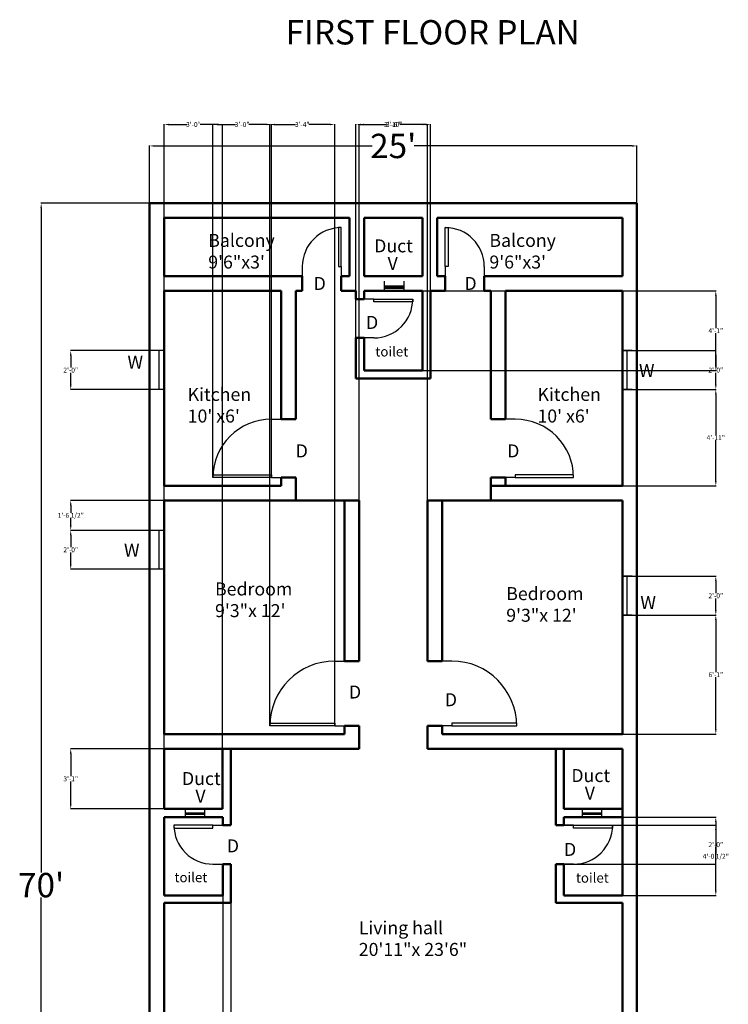
# Model space of a CAD drawing. Units: inches. Extents: x -250 to 2650, y 180 to 1183.
# Tile 4 of 10: x 296 to 732, y 577 to 1183. Entities that reach past the tile are written whole.
import ezdxf

# ---------------------------------------------------------------- set-up
doc = ezdxf.new("R2010")
doc.units = ezdxf.units.IN
doc.header["$MEASUREMENT"] = 0
for name, color, linetype, lineweight in [('A-ANNO-DIMS', 2, 'Continuous', 18), ('A-ANNO-TEXT', 7, 'Continuous', 18), ('A-AREA-IDEN', 3, 'Continuous', 18), ('A-DOOR', 4, 'Continuous', 25), ('A-GLAZ', 3, 'Continuous', 25), ('A-WALL', 7, 'Continuous', 50)]:
    doc.layers.add(name, color=color, linetype=linetype, lineweight=lineweight)
doc.styles.get("Standard").update_dxf_attribs({"font": 'arial.ttf'})
doc.dimstyles.get("Standard").update_dxf_attribs({"dimtxt": 3, "dimasz": 3, "dimexe": 0.18, "dimexo": 0.0625, "dimgap": 0.09, "dimtad": 0, "dimtih": 1, "dimtoh": 1, "dimdec": 0, "dimzin": 0, "dimdsep": 46, "dimlunit": 3, "dimtxsty": 'Standard', "dimcen": 0.09, "dimadec": 0, "dimazin": 0, "dimtfac": 1, "dimtdec": 0, "dimtofl": 0, "dimtmove": 0, "dimatfit": 3, "dimfxl": 1, "dimtolj": 1, "dimtzin": 0, "dimarcsym": 0})

# ---------------------------------------------------------------- blocks, each defined once
blk = doc.blocks.new('*D15')
at = {"layer": 'A-ANNO-DIMS', "color": 0, "lineweight": -2, "transparency": 16777216}
for p, q in [((376.08, 1070.09), (376.08, 1105.5)), ((379.08, 1105.32), (513.14, 1105.32)), ((673.08, 1105.32), (539.03, 1105.32)), ((676.08, 1070.09), (676.08, 1105.5))]:
    blk.add_line(p, q, dxfattribs=at)
at = {"layer": 'A-ANNO-DIMS', "color": 0, "transparency": 16777216}
for points in [[(379.08, 1105.82), (379.08, 1104.82), (376.08, 1105.32)], [(673.08, 1105.82), (673.08, 1104.82), (676.08, 1105.32)]]:
    blk.add_solid(points, dxfattribs=at)
at = {"layer": 'Defpoints', "color": 0, "transparency": 16777216}
for p in [(376.08, 1105.32), (376.08, 1070.02), (676.08, 1070.02)]:
    blk.add_point(p, dxfattribs=at)
at = {"layer": 'A-ANNO-DIMS', "color": 0, "transparency": 16777216, "insert": (526.08, 1105.32), "char_height": 3, "attachment_point": 5}
blk.add_mtext("\\A1;{\\H5x;25'}", dxfattribs=at)
blk = doc.blocks.new('*D16')
at = {"layer": 'A-ANNO-DIMS', "color": 0, "lineweight": -2, "transparency": 16777216}
for p, q in [((376.02, 1070.02), (309.2, 1070.02)), ((309.38, 1067.02), (309.38, 657.77)), ((309.38, 233.02), (309.38, 642.28)), ((376.02, 230.02), (309.2, 230.02))]:
    blk.add_line(p, q, dxfattribs=at)
at = {"layer": 'A-ANNO-DIMS', "color": 0, "transparency": 16777216}
for points in [[(308.88, 1067.02), (309.88, 1067.02), (309.38, 1070.02)], [(308.88, 233.02), (309.88, 233.02), (309.38, 230.02)]]:
    blk.add_solid(points, dxfattribs=at)
at = {"layer": 'Defpoints', "color": 0, "transparency": 16777216}
for p in [(376.08, 1070.02), (309.38, 230.02), (376.08, 230.02)]:
    blk.add_point(p, dxfattribs=at)
at = {"layer": 'A-ANNO-DIMS', "color": 0, "transparency": 16777216, "insert": (309.38, 650.02), "char_height": 3, "attachment_point": 5}
blk.add_mtext("\\A1;{\\H5x;70'}", dxfattribs=at)
blk = doc.blocks.new('*U17')
for p, q in [((-24, 0), (-24, -6)), ((0, 0), (0, -6))]:
    blk.add_line(p, q)
blk.add_lwpolyline([(0, 0), (0, 24), (-1.75, 24), (-1.75, 0)], close=True)
blk.add_arc((0, 0), 24, 90, 180)
blk = doc.blocks.new('*U18')
for p, q in [((0, 0), (0, -6)), ((24, 0), (24, -6))]:
    blk.add_line(p, q)
blk.add_lwpolyline([(0, 0), (0, 24), (1.75, 24), (1.75, 0)], close=True)
blk.add_arc((0, 0), 24, 0, 90)
blk = doc.blocks.new('*U19')
for p, q in [((0, 0), (0, -6)), ((24, 0), (24, -6))]:
    blk.add_line(p, q)
blk.add_lwpolyline([(0, 0), (0, 24), (1.75, 24), (1.75, 0)], close=True)
blk.add_arc((0, 0), 24, 0, 90)
blk = doc.blocks.new('*U20')
for p, q in [((-36, 0), (-36, -6)), ((0, 0), (0, -6))]:
    blk.add_line(p, q)
blk.add_lwpolyline([(0, 0), (0, 36), (-1.75, 36), (-1.75, 0)], close=True)
blk.add_arc((0, 0), 36, 90, 180)
blk = doc.blocks.new('*U21')
for p, q in [((-36, 0), (-36, 6)), ((0, 0), (0, 6))]:
    blk.add_line(p, q)
blk.add_lwpolyline([(0, 0), (0, -36), (-1.75, -36), (-1.75, 0)], close=True)
blk.add_arc((0, 0), 36, 180, 270)
blk = doc.blocks.new('*U24')
for p, q in [((-24, 6), (-24, 0)), ((0, 3), (-24, 3)), ((0, 6), (0, 0))]:
    blk.add_line(p, q)
blk = doc.blocks.new('*U23')
for p, q in [((-24, 6), (-24, 0)), ((0, 3), (-24, 3)), ((0, 6), (0, 0))]:
    blk.add_line(p, q)
blk = doc.blocks.new('*U22')
for p, q in [((0, 6), (0, 0)), ((0, 3), (12, 3)), ((12, 6), (12, 0))]:
    blk.add_line(p, q)
blk = doc.blocks.new('*U25')
for p, q in [((-40, 0), (-40, 6)), ((0, 0), (0, 6))]:
    blk.add_line(p, q)
blk.add_lwpolyline([(0, 0), (0, -40), (-1.75, -40), (-1.75, 0)], close=True)
blk.add_arc((0, 0), 40, 180, 270)
blk = doc.blocks.new('*U26')
for p, q in [((-40, 0), (-40, -6)), ((0, 0), (0, -6))]:
    blk.add_line(p, q)
blk.add_lwpolyline([(0, 0), (0, 40), (-1.75, 40), (-1.75, 0)], close=True)
blk.add_arc((0, 0), 40, 90, 180)
blk = doc.blocks.new('*U27')
for p, q in [((0, 0), (0, -6)), ((24, 0), (24, -6))]:
    blk.add_line(p, q)
blk.add_lwpolyline([(0, 0), (0, 24), (1.75, 24), (1.75, 0)], close=True)
blk.add_arc((0, 0), 24, 0, 90)
blk = doc.blocks.new('*U28')
for p, q in [((0, 0), (0, 6)), ((24, 0), (24, 6))]:
    blk.add_line(p, q)
blk.add_lwpolyline([(0, 0), (0, -24), (1.75, -24), (1.75, 0)], close=True)
blk.add_arc((0, 0), 24, 270, 0)
blk = doc.blocks.new('*U29')
for p, q in [((0, 5), (0, 0)), ((0, 2.5), (12, 2.5)), ((12, 5), (12, 0))]:
    blk.add_line(p, q)
blk = doc.blocks.new('*D81')
at = {"layer": 'A-ANNO-DIMS', "color": 0, "lineweight": -2, "transparency": 16777216}
for p, q in [((385.08, 734.09), (385.08, 1118.7)), ((388.08, 1118.52), (399.01, 1118.52)), ((418.08, 1118.52), (407.16, 1118.52)), ((421.08, 734.09), (421.08, 1118.7))]:
    blk.add_line(p, q, dxfattribs=at)
at = {"layer": 'A-ANNO-DIMS', "color": 0, "transparency": 16777216}
for points in [[(388.08, 1119.02), (388.08, 1118.02), (385.08, 1118.52)], [(418.08, 1119.02), (418.08, 1118.02), (421.08, 1118.52)]]:
    blk.add_solid(points, dxfattribs=at)
at = {"layer": 'Defpoints', "color": 0, "transparency": 16777216}
for p in [(421.08, 1118.52), (385.08, 734.02), (421.08, 734.02)]:
    blk.add_point(p, dxfattribs=at)
at = {"layer": 'A-ANNO-DIMS', "color": 0, "transparency": 16777216, "insert": (403.08, 1118.52), "char_height": 3, "attachment_point": 5}
blk.add_mtext('\\A1;3\'-0"', dxfattribs=at)
blk = doc.blocks.new('*D82')
at = {"layer": 'A-ANNO-DIMS', "color": 0, "lineweight": -2, "transparency": 16777216}
for p, q in [((421.09, 643.56), (421.09, 181.34)), ((426.08, 639.05), (426.08, 181.34)), ((418.09, 181.52), (415.09, 181.52)), ((429.08, 181.52), (432.08, 181.52))]:
    blk.add_line(p, q, dxfattribs=at)
at = {"layer": 'A-ANNO-DIMS', "color": 0, "transparency": 16777216}
for points in [[(418.09, 182.02), (418.09, 181.02), (421.09, 181.52)], [(429.08, 182.02), (429.08, 181.02), (426.08, 181.52)]]:
    blk.add_solid(points, dxfattribs=at)
at = {"layer": 'Defpoints', "color": 0, "transparency": 16777216}
for p in [(421.09, 643.62), (426.08, 639.11), (426.08, 181.52)]:
    blk.add_point(p, dxfattribs=at)
at = {"layer": 'A-ANNO-DIMS', "color": 0, "transparency": 16777216, "insert": (436.16, 181.52), "char_height": 3, "attachment_point": 5}
blk.add_mtext('\\A1;0\'-5"', dxfattribs=at)
blk = doc.blocks.new('*D83')
at = {"layer": 'A-ANNO-DIMS', "color": 0, "lineweight": -2, "transparency": 16777216}
for p, q in [((385.02, 734.02), (327.4, 734.02)), ((327.58, 731.02), (327.58, 717.09)), ((327.58, 699.91), (327.58, 713.84)), ((385.02, 696.91), (327.4, 696.91))]:
    blk.add_line(p, q, dxfattribs=at)
at = {"layer": 'A-ANNO-DIMS', "color": 0, "transparency": 16777216}
for points in [[(327.08, 731.02), (328.08, 731.02), (327.58, 734.02)], [(327.08, 699.91), (328.08, 699.91), (327.58, 696.91)]]:
    blk.add_solid(points, dxfattribs=at)
at = {"layer": 'Defpoints', "color": 0, "transparency": 16777216}
for p in [(327.58, 734.02), (385.08, 734.02), (385.08, 696.91)]:
    blk.add_point(p, dxfattribs=at)
at = {"layer": 'A-ANNO-DIMS', "color": 0, "transparency": 16777216, "insert": (327.58, 715.47), "char_height": 3, "attachment_point": 5}
blk.add_mtext('\\A1;3\'-1"', dxfattribs=at)
blk = doc.blocks.new('*D84')
at = {"layer": 'A-ANNO-DIMS', "color": 0, "lineweight": -2, "transparency": 16777216}
for p, q in [((667.15, 691.91), (724.76, 691.91)), ((724.58, 688.91), (724.58, 669.41)), ((724.58, 646.62), (724.58, 666.12)), ((667.15, 643.62), (724.76, 643.62))]:
    blk.add_line(p, q, dxfattribs=at)
at = {"layer": 'A-ANNO-DIMS', "color": 0, "transparency": 16777216}
for points in [[(724.08, 688.91), (725.08, 688.91), (724.58, 691.91)], [(724.08, 646.62), (725.08, 646.62), (724.58, 643.62)]]:
    blk.add_solid(points, dxfattribs=at)
at = {"layer": 'Defpoints', "color": 0, "transparency": 16777216}
for p in [(667.08, 691.91), (724.58, 691.91), (667.08, 643.62)]:
    blk.add_point(p, dxfattribs=at)
at = {"layer": 'A-ANNO-DIMS', "color": 0, "transparency": 16777216, "insert": (724.58, 667.77), "char_height": 3, "attachment_point": 5}
blk.add_mtext('\\A1;4\'-0 1/2"', dxfattribs=at)
blk = doc.blocks.new('*D90')
at = {"layer": 'A-ANNO-DIMS', "color": 0, "lineweight": -2, "transparency": 16777216}
for p, q in [((626.15, 686.91), (724.76, 686.91)), ((724.58, 683.91), (724.58, 676.53)), ((724.58, 665.91), (724.58, 673.29)), ((626.15, 662.91), (724.76, 662.91))]:
    blk.add_line(p, q, dxfattribs=at)
at = {"layer": 'A-ANNO-DIMS', "color": 0, "transparency": 16777216}
for points in [[(724.08, 683.91), (725.08, 683.91), (724.58, 686.91)], [(724.08, 665.91), (725.08, 665.91), (724.58, 662.91)]]:
    blk.add_solid(points, dxfattribs=at)
at = {"layer": 'Defpoints', "color": 0, "transparency": 16777216}
for p in [(626.08, 686.91), (724.58, 686.91), (626.08, 662.91)]:
    blk.add_point(p, dxfattribs=at)
at = {"layer": 'A-ANNO-DIMS', "color": 0, "transparency": 16777216, "insert": (724.58, 674.91), "char_height": 3, "attachment_point": 5}
blk.add_mtext('\\A1;2\'-0"', dxfattribs=at)
blk = doc.blocks.new('*D91')
at = {"layer": 'A-ANNO-DIMS', "color": 0, "lineweight": -2, "transparency": 16777216}
for p, q in [((505.08, 887.09), (505.08, 1118.7)), ((508.08, 1118.52), (522.01, 1118.52)), ((544.08, 1118.52), (530.16, 1118.52)), ((547.08, 887.09), (547.08, 1118.7))]:
    blk.add_line(p, q, dxfattribs=at)
at = {"layer": 'A-ANNO-DIMS', "color": 0, "transparency": 16777216}
for points in [[(508.08, 1119.02), (508.08, 1118.02), (505.08, 1118.52)], [(544.08, 1119.02), (544.08, 1118.02), (547.08, 1118.52)]]:
    blk.add_solid(points, dxfattribs=at)
at = {"layer": 'Defpoints', "color": 0, "transparency": 16777216}
for p in [(547.08, 1118.52), (505.08, 887.02), (547.08, 887.02)]:
    blk.add_point(p, dxfattribs=at)
at = {"layer": 'A-ANNO-DIMS', "color": 0, "transparency": 16777216, "insert": (526.08, 1118.52), "char_height": 3, "attachment_point": 5}
blk.add_mtext('\\A1;3\'-6"', dxfattribs=at)
blk = doc.blocks.new('*D92')
at = {"layer": 'A-ANNO-DIMS', "color": 0, "lineweight": -2, "transparency": 16777216}
for p, q in [((503.08, 962.09), (503.08, 1118.7)), ((506.08, 1118.52), (520.84, 1118.52)), ((546.08, 1118.52), (531.33, 1118.52)), ((549.08, 962.09), (549.08, 1118.7))]:
    blk.add_line(p, q, dxfattribs=at)
at = {"layer": 'A-ANNO-DIMS', "color": 0, "transparency": 16777216}
for points in [[(506.08, 1119.02), (506.08, 1118.02), (503.08, 1118.52)], [(546.08, 1119.02), (546.08, 1118.02), (549.08, 1118.52)]]:
    blk.add_solid(points, dxfattribs=at)
at = {"layer": 'Defpoints', "color": 0, "transparency": 16777216}
for p in [(549.08, 1118.52), (503.08, 962.02), (549.08, 962.02)]:
    blk.add_point(p, dxfattribs=at)
at = {"layer": 'A-ANNO-DIMS', "color": 0, "transparency": 16777216, "insert": (526.08, 1118.52), "char_height": 3, "attachment_point": 5}
blk.add_mtext('\\A1;3\'-10"', dxfattribs=at)
blk = doc.blocks.new('*D93')
at = {"layer": 'A-ANNO-DIMS', "color": 0, "lineweight": -2, "transparency": 16777216}
for p, q in [((544.15, 1016.02), (724.76, 1016.02)), ((724.58, 1013.02), (724.58, 993.12)), ((724.58, 970.02), (724.58, 989.93)), ((544.15, 967.02), (724.76, 967.02))]:
    blk.add_line(p, q, dxfattribs=at)
at = {"layer": 'A-ANNO-DIMS', "color": 0, "transparency": 16777216}
for points in [[(724.08, 1013.02), (725.08, 1013.02), (724.58, 1016.02)], [(724.08, 970.02), (725.08, 970.02), (724.58, 967.02)]]:
    blk.add_solid(points, dxfattribs=at)
at = {"layer": 'Defpoints', "color": 0, "transparency": 16777216}
for p in [(544.08, 1016.02), (544.08, 967.02), (724.58, 967.02)]:
    blk.add_point(p, dxfattribs=at)
at = {"layer": 'A-ANNO-DIMS', "color": 0, "transparency": 16777216, "insert": (724.58, 991.52), "char_height": 3, "attachment_point": 5}
blk.add_mtext('\\A1;4\'-1"', dxfattribs=at)
blk = doc.blocks.new('*D94')
at = {"layer": 'A-ANNO-DIMS', "color": 0, "lineweight": -2, "transparency": 16777216}
for p, q in [((667.15, 816.25), (724.76, 816.25)), ((724.58, 813.25), (724.58, 781.26)), ((724.58, 746.02), (724.58, 778.01)), ((667.15, 743.02), (724.76, 743.02))]:
    blk.add_line(p, q, dxfattribs=at)
at = {"layer": 'A-ANNO-DIMS', "color": 0, "transparency": 16777216}
for points in [[(724.08, 813.25), (725.08, 813.25), (724.58, 816.25)], [(724.08, 746.02), (725.08, 746.02), (724.58, 743.02)]]:
    blk.add_solid(points, dxfattribs=at)
at = {"layer": 'Defpoints', "color": 0, "transparency": 16777216}
for p in [(667.08, 816.25), (724.58, 816.25), (667.08, 743.02)]:
    blk.add_point(p, dxfattribs=at)
at = {"layer": 'A-ANNO-DIMS', "color": 0, "transparency": 16777216, "insert": (724.58, 779.64), "char_height": 3, "attachment_point": 5}
blk.add_mtext('\\A1;6\'-1"', dxfattribs=at)
blk = doc.blocks.new('*D95')
at = {"layer": 'A-ANNO-DIMS', "color": 0, "lineweight": -2, "transparency": 16777216}
for p, q in [((667.15, 840.25), (724.76, 840.25)), ((724.58, 837.25), (724.58, 829.87)), ((724.58, 819.25), (724.58, 826.63)), ((667.15, 816.25), (724.76, 816.25))]:
    blk.add_line(p, q, dxfattribs=at)
at = {"layer": 'A-ANNO-DIMS', "color": 0, "transparency": 16777216}
for points in [[(724.08, 837.25), (725.08, 837.25), (724.58, 840.25)], [(724.08, 819.25), (725.08, 819.25), (724.58, 816.25)]]:
    blk.add_solid(points, dxfattribs=at)
at = {"layer": 'Defpoints', "color": 0, "transparency": 16777216}
for p in [(667.08, 840.25), (724.58, 840.25), (667.08, 816.25)]:
    blk.add_point(p, dxfattribs=at)
at = {"layer": 'A-ANNO-DIMS', "color": 0, "transparency": 16777216, "insert": (724.58, 828.25), "char_height": 3, "attachment_point": 5}
blk.add_mtext('\\A1;2\'-0"', dxfattribs=at)
blk = doc.blocks.new('*D96')
at = {"layer": 'A-ANNO-DIMS', "color": 0, "lineweight": -2, "transparency": 16777216}
for p, q in [((667.15, 955.23), (724.76, 955.23)), ((724.58, 952.23), (724.58, 927.22)), ((724.58, 899.02), (724.58, 924.03)), ((667.15, 896.02), (724.76, 896.02))]:
    blk.add_line(p, q, dxfattribs=at)
at = {"layer": 'A-ANNO-DIMS', "color": 0, "transparency": 16777216}
for points in [[(724.08, 952.23), (725.08, 952.23), (724.58, 955.23)], [(724.08, 899.02), (725.08, 899.02), (724.58, 896.02)]]:
    blk.add_solid(points, dxfattribs=at)
at = {"layer": 'Defpoints', "color": 0, "transparency": 16777216}
for p in [(667.08, 955.23), (724.58, 955.23), (667.08, 896.02)]:
    blk.add_point(p, dxfattribs=at)
at = {"layer": 'A-ANNO-DIMS', "color": 0, "transparency": 16777216, "insert": (724.58, 925.63), "char_height": 3, "attachment_point": 5}
blk.add_mtext('\\A1;4\'-11"', dxfattribs=at)
blk = doc.blocks.new('*D97')
at = {"layer": 'A-ANNO-DIMS', "color": 0, "lineweight": -2, "transparency": 16777216}
for p, q in [((667.15, 979.23), (724.76, 979.23)), ((724.58, 976.23), (724.58, 968.85)), ((724.58, 958.23), (724.58, 965.61)), ((667.15, 955.23), (724.76, 955.23))]:
    blk.add_line(p, q, dxfattribs=at)
at = {"layer": 'A-ANNO-DIMS', "color": 0, "transparency": 16777216}
for points in [[(724.08, 976.23), (725.08, 976.23), (724.58, 979.23)], [(724.08, 958.23), (725.08, 958.23), (724.58, 955.23)]]:
    blk.add_solid(points, dxfattribs=at)
at = {"layer": 'Defpoints', "color": 0, "transparency": 16777216}
for p in [(667.08, 979.23), (724.58, 979.23), (667.08, 955.23)]:
    blk.add_point(p, dxfattribs=at)
at = {"layer": 'A-ANNO-DIMS', "color": 0, "transparency": 16777216, "insert": (724.58, 967.23), "char_height": 3, "attachment_point": 5}
blk.add_mtext('\\A1;2\'-0"', dxfattribs=at)
blk = doc.blocks.new('*D98')
at = {"layer": 'A-ANNO-DIMS', "color": 0, "lineweight": -2, "transparency": 16777216}
for p, q in [((385.02, 868.53), (327.4, 868.53)), ((327.58, 865.53), (327.58, 858.15)), ((327.58, 847.53), (327.58, 854.91)), ((385.02, 844.53), (327.4, 844.53))]:
    blk.add_line(p, q, dxfattribs=at)
at = {"layer": 'A-ANNO-DIMS', "color": 0, "transparency": 16777216}
for points in [[(327.08, 865.53), (328.08, 865.53), (327.58, 868.53)], [(327.08, 847.53), (328.08, 847.53), (327.58, 844.53)]]:
    blk.add_solid(points, dxfattribs=at)
at = {"layer": 'Defpoints', "color": 0, "transparency": 16777216}
for p in [(327.58, 868.53), (385.08, 868.53), (385.08, 844.53)]:
    blk.add_point(p, dxfattribs=at)
at = {"layer": 'A-ANNO-DIMS', "color": 0, "transparency": 16777216, "insert": (327.58, 856.53), "char_height": 3, "attachment_point": 5}
blk.add_mtext('\\A1;2\'-0"', dxfattribs=at)
blk = doc.blocks.new('*D99')
at = {"layer": 'A-ANNO-DIMS', "color": 0, "lineweight": -2, "transparency": 16777216}
for p, q in [((385.02, 887.02), (327.4, 887.02)), ((327.58, 884.02), (327.58, 879.42)), ((327.58, 871.53), (327.58, 876.14)), ((385.02, 868.53), (327.4, 868.53))]:
    blk.add_line(p, q, dxfattribs=at)
at = {"layer": 'A-ANNO-DIMS', "color": 0, "transparency": 16777216}
for points in [[(327.08, 884.02), (328.08, 884.02), (327.58, 887.02)], [(327.08, 871.53), (328.08, 871.53), (327.58, 868.53)]]:
    blk.add_solid(points, dxfattribs=at)
at = {"layer": 'Defpoints', "color": 0, "transparency": 16777216}
for p in [(327.58, 887.02), (385.08, 887.02), (385.08, 868.53)]:
    blk.add_point(p, dxfattribs=at)
at = {"layer": 'A-ANNO-DIMS', "color": 0, "transparency": 16777216, "insert": (327.58, 877.78), "char_height": 3, "attachment_point": 5}
blk.add_mtext('\\A1;1\'-6 1/2"', dxfattribs=at)
blk = doc.blocks.new('*D100')
at = {"layer": 'A-ANNO-DIMS', "color": 0, "lineweight": -2, "transparency": 16777216}
for p, q in [((385.02, 979.23), (327.4, 979.23)), ((327.58, 976.23), (327.58, 968.85)), ((327.58, 958.23), (327.58, 965.61)), ((385.02, 955.23), (327.4, 955.23))]:
    blk.add_line(p, q, dxfattribs=at)
at = {"layer": 'A-ANNO-DIMS', "color": 0, "transparency": 16777216}
for points in [[(327.08, 976.23), (328.08, 976.23), (327.58, 979.23)], [(327.08, 958.23), (328.08, 958.23), (327.58, 955.23)]]:
    blk.add_solid(points, dxfattribs=at)
at = {"layer": 'Defpoints', "color": 0, "transparency": 16777216}
for p in [(327.58, 979.23), (385.08, 979.23), (385.08, 955.23)]:
    blk.add_point(p, dxfattribs=at)
at = {"layer": 'A-ANNO-DIMS', "color": 0, "transparency": 16777216, "insert": (327.58, 967.23), "char_height": 3, "attachment_point": 5}
blk.add_mtext('\\A1;2\'-0"', dxfattribs=at)
blk = doc.blocks.new('*D101')
at = {"layer": 'A-ANNO-DIMS', "color": 0, "lineweight": -2, "transparency": 16777216}
for p, q in [((450.08, 748.09), (450.08, 1118.7)), ((453.08, 1118.52), (466.01, 1118.52)), ((487.08, 1118.52), (474.16, 1118.52)), ((490.08, 748.09), (490.08, 1118.7))]:
    blk.add_line(p, q, dxfattribs=at)
at = {"layer": 'A-ANNO-DIMS', "color": 0, "transparency": 16777216}
for points in [[(453.08, 1119.02), (453.08, 1118.02), (450.08, 1118.52)], [(487.08, 1119.02), (487.08, 1118.02), (490.08, 1118.52)]]:
    blk.add_solid(points, dxfattribs=at)
at = {"layer": 'Defpoints', "color": 0, "transparency": 16777216}
for p in [(490.08, 1118.52), (450.08, 748.02), (490.08, 748.02)]:
    blk.add_point(p, dxfattribs=at)
at = {"layer": 'A-ANNO-DIMS', "color": 0, "transparency": 16777216, "insert": (470.08, 1118.52), "char_height": 3, "attachment_point": 5}
blk.add_mtext('\\A1;3\'-4"', dxfattribs=at)
blk = doc.blocks.new('*D102')
at = {"layer": 'A-ANNO-DIMS', "color": 0, "lineweight": -2, "transparency": 16777216}
for p, q in [((415.08, 901.09), (415.08, 1118.7)), ((418.08, 1118.52), (429.01, 1118.52)), ((448.08, 1118.52), (437.16, 1118.52)), ((451.08, 901.09), (451.08, 1118.7))]:
    blk.add_line(p, q, dxfattribs=at)
at = {"layer": 'A-ANNO-DIMS', "color": 0, "transparency": 16777216}
for points in [[(418.08, 1119.02), (418.08, 1118.02), (415.08, 1118.52)], [(448.08, 1119.02), (448.08, 1118.02), (451.08, 1118.52)]]:
    blk.add_solid(points, dxfattribs=at)
at = {"layer": 'Defpoints', "color": 0, "transparency": 16777216}
for p in [(451.08, 1118.52), (415.08, 901.02), (451.08, 901.02)]:
    blk.add_point(p, dxfattribs=at)
at = {"layer": 'A-ANNO-DIMS', "color": 0, "transparency": 16777216, "insert": (433.08, 1118.52), "char_height": 3, "attachment_point": 5}
blk.add_mtext('\\A1;3\'-0"', dxfattribs=at)

msp = doc.modelspace()

# ---------------------------------------------------------------- linework, layer by layer
at = {"layer": 'A-WALL'}
for p, q in [((676.08, 1070.02), (376.08, 1070.02)), ((376.08, 1070.02), (376.08, 230.02)), ((676.08, 230.02), (676.08, 1070.02)), ((385.08, 1061.02), (385.08, 1025.02)), ((499.08, 1061.02), (385.08, 1061.02)), ((499.08, 1061.02), (499.08, 1025.02)), ((544.08, 1061.02), (508.08, 1061.02)), ((508.08, 1061.02), (508.08, 1025.02)), ((544.08, 1025.02), (544.08, 1061.02)), ((667.08, 1061.02), (553.08, 1061.02)), ((553.08, 1025.02), (553.08, 1061.02)), ((667.08, 1025.02), (667.08, 1061.02)), ((667.08, 1025.02), (667.08, 1061.02)), ((667.08, 1025.02), (667.08, 1061.02)), ((667.08, 1025.02), (667.08, 1061.02)), ((470.08, 1025.02), (385.08, 1025.02)), ((470.08, 1025.02), (470.08, 1016.02)), ((499.08, 1025.02), (494.08, 1025.02)), ((494.08, 1016.02), (494.08, 1025.02)), ((544.08, 1025.02), (508.08, 1025.02)), ((558.08, 1025.02), (553.08, 1025.02)), ((558.08, 1016.02), (558.08, 1025.02)), ((582.08, 1025.02), (582.08, 1016.02)), ((667.08, 1025.02), (582.08, 1025.02)), ((385.08, 1016.02), (385.08, 896.02)), ((457.08, 1016.02), (385.08, 1016.02)), ((457.08, 1016.02), (457.08, 937.02)), ((466.08, 1016.02), (466.08, 937.02)), ((470.08, 1016.02), (466.08, 1016.02)), ((503.08, 1016.02), (494.08, 1016.02)), ((503.08, 1016.02), (503.08, 1011.02)), ((508.08, 1016.03), (508.08, 1011.02)), ((544.08, 1016.02), (508.08, 1016.02)), ((532.77, 1017.95), (520.77, 1017.95)), ((544.08, 967.02), (544.08, 1016.02)), ((549.08, 962.02), (549.08, 1016.02)), ((558.08, 1016.02), (549.08, 1016.02)), ((586.08, 1016.02), (582.08, 1016.02)), ((586.08, 937.02), (586.08, 1016.02)), ((595.08, 937.02), (595.08, 1016.02)), ((667.08, 1016.02), (595.08, 1016.02)), ((667.08, 896.02), (667.08, 1016.02)), ((667.08, 896.02), (667.08, 1016.02)), ((667.08, 896.02), (667.08, 1016.02)), ((508.08, 1011.02), (503.08, 1011.02)), ((508.08, 987.02), (503.08, 987.02)), ((503.08, 987.02), (503.08, 962.02)), ((508.08, 987.02), (508.08, 967.02)), ((544.08, 967.02), (508.08, 967.02)), ((549.08, 962.02), (503.08, 962.02)), ((457.08, 937.02), (466.08, 937.02)), ((595.08, 937.02), (586.08, 937.02)), ((457.08, 901.02), (466.08, 901.02)), ((457.08, 901.02), (457.08, 896.02)), ((466.08, 901.02), (466.08, 887.02)), ((586.08, 887.02), (586.08, 901.02)), ((595.08, 901.02), (586.08, 901.02)), ((595.08, 896.02), (595.08, 901.02)), ((457.08, 896.02), (385.08, 896.02)), ((667.08, 896.02), (586.08, 896.02)), ((385.08, 887.02), (385.08, 743.02)), ((505.08, 887.02), (385.08, 887.02)), ((496.08, 887.02), (496.08, 788.02)), ((505.08, 887.02), (505.08, 788.02)), ((547.08, 788.02), (547.08, 887.02)), ((667.08, 887.02), (547.08, 887.02)), ((556.08, 788.02), (556.08, 887.02)), ((667.08, 743.02), (667.08, 887.02)), ((667.08, 743.02), (667.08, 887.02)), ((667.08, 743.02), (667.08, 887.02)), ((496.08, 788.02), (505.08, 788.02)), ((556.08, 788.02), (547.08, 788.02)), ((496.08, 748.02), (505.08, 748.02)), ((496.08, 748.02), (496.08, 743.02)), ((505.08, 748.02), (505.08, 734.02)), ((556.08, 748.02), (547.08, 748.02)), ((547.08, 748.02), (547.08, 734.02)), ((556.08, 743.02), (556.08, 748.02)), ((496.08, 743.02), (385.08, 743.02)), ((667.08, 743.02), (556.08, 743.02)), ((505.08, 734.02), (385.08, 734.02)), ((385.08, 734.02), (385.08, 696.91)), ((421.08, 696.91), (421.08, 734.02)), ((426.08, 686.91), (426.08, 734.02)), ((667.08, 734.02), (547.08, 734.02)), ((626.08, 686.91), (626.08, 734.02)), ((626.08, 686.91), (626.08, 734.02)), ((631.08, 696.91), (631.08, 734.02)), ((667.08, 716.02), (667.08, 734.02)), ((667.08, 696.91), (667.08, 734.02)), ((667.08, 643.62), (667.08, 734.02)), ((421.08, 696.91), (385.08, 696.91)), ((421.09, 691.91), (385.08, 691.91)), ((385.08, 691.91), (385.08, 643.62)), ((410.14, 693.93), (398.14, 693.93)), ((421.09, 691.91), (421.09, 686.91)), ((667.08, 696.91), (631.08, 696.91)), ((667.08, 691.91), (631.08, 691.91)), ((631.08, 686.91), (631.08, 691.91)), ((654.52, 693.93), (642.52, 693.93)), ((667.08, 643.62), (667.08, 691.91)), ((421.09, 686.91), (426.08, 686.91)), ((631.08, 686.91), (626.08, 686.91)), ((421.09, 662.91), (426.09, 662.91)), ((421.09, 662.91), (421.09, 643.62)), ((426.08, 639.11), (426.08, 662.91)), ((426.09, 662.91), (426.09, 639.11)), ((626.08, 639.11), (626.08, 662.91)), ((626.08, 643.62), (626.08, 662.91)), ((631.08, 662.91), (626.08, 662.91)), ((631.08, 643.62), (631.08, 662.91)), ((421.09, 643.62), (385.08, 643.62)), ((426.09, 643.62), (426.08, 643.62)), ((667.08, 643.62), (631.08, 643.62)), ((426.09, 639.11), (385.08, 639.11)), ((385.08, 639.11), (385.08, 483.11)), ((667.08, 639.11), (626.08, 639.11)), ((667.08, 587.02), (667.08, 639.11)), ((667.08, 483.11), (667.08, 639.11))]:
    msp.add_line(p, q, dxfattribs=at)

# ---------------------------------------------------------------- block references
at = {"layer": 'A-DOOR'}
for name, p in [('*U17', (494.08, 1031.02)), ('*U18', (558.08, 1031.02))]:
    msp.add_blockref(name, p, dxfattribs=at)
at = {"layer": 'A-DOOR', "rotation": 270}
for name, p in [('*U19', (514.08, 1011.02)), ('*U21', (451.08, 901.02)), ('*U20', (601.08, 901.02)), ('*U25', (490.08, 748.02)), ('*U26', (562.08, 748.02)), ('*U28', (415.09, 686.91)), ('*U27', (637.08, 686.91))]:
    msp.add_blockref(name, p, dxfattribs=at)
at = {"layer": 'A-GLAZ'}
for name, p, rotation in [('*U22', (532.77, 1021.95), 180), ('*U23', (379.08, 955.23), 270), ('*U24', (667.08, 955.23), 270), ('*U23', (379.08, 844.53), 270), ('*U24', (667.08, 816.25), 270), ('*U29', (410.14, 696.91), 180), ('*U29', (654.52, 696.91), 180)]:
    msp.add_blockref(name, p, dxfattribs=dict(at, rotation=rotation))

# ---------------------------------------------------------------- texts
at = {"layer": 'A-ANNO-TEXT', "attachment_point": 1}
for s, width, insert, char_height in [('FIRST FLOOR PLAN ', 207.4062, (459.89, 1182.82), 15), ('V', 10.3916, (522.59, 1036.98), 8), ('D', 10.3916, (477.07, 1024.6), 8), ('D', 10.3916, (569.88, 1024.6), 8), ('D', 10.3916, (509.32, 1000.62), 8), ('W', 10.3916, (362.5, 976.14), 8), ('W', 10.3916, (362.5, 976.14), 8), ('W', 10.3916, (677.27, 971.03), 8), ('D', 10.3916, (466.03, 921.46), 8), ('D', 10.3916, (596.21, 921.46), 8), ('W', 10.3916, (360.35, 860.33), 8), ('W', 10.3916, (678.15, 828), 8), ('D', 10.3916, (498.82, 772.95), 8), ('D', 10.3916, (557.81, 768.2), 8), ('V', 10.3916, (643.95, 710.71), 8), ('V', 10.3916, (404.31, 708.86), 8), ('D', 10.3916, (423.66, 678.19), 8), ('D', 10.3916, (631.17, 675.98), 8)]:
    msp.add_mtext_dynamic_manual_height_columns(s, width=width, gutter_width=1, heights=[0], dxfattribs=dict(at, insert=insert, char_height=char_height))
at = {"layer": 'A-AREA-IDEN', "attachment_point": 1}
for s, width, heights, insert, char_height in [('Balcony 9\'6"x3\'', 37.1044, [0], (412.22, 1051.13), 8), ('Balcony 9\'6"x3\'', 37.1044, [0], (585.24, 1051.13), 8), ('{\\H2.66667x;Duct} ', 7.71, [3.05], (514.34, 1047.76), 3), ('toilet', 19.3499, [0], (515.05, 981.65), 6), ("Kitchen 10' x6'", 37.1044, [0], (399.55, 956.28), 8), ("Kitchen 10' x6'", 37.1044, [0], (614.82, 956.28), 8), ('Bedroom \\P9\'3"x 12\'', 51.3886, [0], (416.4, 836.41), 8), ('Bedroom \\P9\'3"x 12\'', 51.3886, [0], (595.6, 833.56), 8), ('{\\H2.66667x;Duct} ', 7.71, [3.05], (396.05, 719.65), 3), ('{\\H2.66667x;Duct} ', 7.71, [3.05], (635.7, 721.49), 3), ('toilet', 19.3499, [0], (391.43, 657.78), 6), ('toilet', 19.3499, [0], (638.47, 657.5), 6), ('Living hall  \\P20\'11"x 23\'6"', 123.5412, [0], (504.85, 627.72), 8)]:
    msp.add_mtext_dynamic_manual_height_columns(s, width=width, gutter_width=1, heights=heights, dxfattribs=dict(at, insert=insert, char_height=char_height))

# ---------------------------------------------------------------- dimensions: what is measured, and where the dimension line sits
at = {"layer": 'A-ANNO-DIMS'}
for base, p1, p2, picture, middle in [((421.08, 1118.52), (385.08, 734.02), (421.08, 734.02), '*D81', (403.08, 1118.52)), ((451.08, 1118.52), (415.08, 901.02), (451.08, 901.02), '*D102', (433.08, 1118.52)), ((490.08, 1118.52), (450.08, 748.02), (490.08, 748.02), '*D101', (470.08, 1118.52)), ((549.08, 1118.52), (503.08, 962.02), (549.08, 962.02), '*D92', (526.08, 1118.52)), ((547.08, 1118.52), (505.08, 887.02), (547.08, 887.02), '*D91', (526.08, 1118.52)), ((426.08, 181.52), (421.09, 643.62), (426.08, 639.11), '*D82', (436.16, 181.52))]:
    dim = msp.add_linear_dim(base=base, p1=p1, p2=p2, dimstyle='Standard', override={"dimdec": 1, "dimlfac": 1, "dimrnd": 0, "dimzin": 1, "dimdsep": 46, "dimlunit": 4, "dimfrac": 2}, dxfattribs=at)
    dim.commit()
    dim.dimension.update_dxf_attribs({"geometry": picture, "text_midpoint": middle})
dim = msp.add_linear_dim(base=(376.08, 1105.32), p1=(676.08, 1070.02), p2=(376.08, 1070.02), text='{\\H5x;<>}', dimstyle='Standard', override={"dimclrd": 0, "dimclre": 0, "dimclrt": 0}, dxfattribs=at)
dim.commit()
dim.dimension.update_dxf_attribs({"geometry": '*D15', "text_midpoint": (526.08, 1105.32)})
dim = msp.add_linear_dim(base=(309.38, 230.02), p1=(376.08, 1070.02), p2=(376.08, 230.02), angle=90, text='{\\H5x;<>}', dimstyle='Standard', override={"dimclrd": 0, "dimclre": 0, "dimclrt": 0}, dxfattribs=at)
dim.commit()
dim.dimension.update_dxf_attribs({"geometry": '*D16', "text_midpoint": (309.38, 650.02)})
for base, p1, p2, picture, middle in [((724.58, 967.02), (544.08, 1016.02), (544.08, 967.02), '*D93', (724.58, 991.52)), ((327.58, 979.23), (385.08, 955.23), (385.08, 979.23), '*D100', (327.58, 967.23)), ((724.58, 979.23), (667.08, 955.23), (667.08, 979.23), '*D97', (724.58, 967.23)), ((724.58, 955.23), (667.08, 896.02), (667.08, 955.23), '*D96', (724.58, 925.63)), ((327.58, 887.02), (385.08, 868.53), (385.08, 887.02), '*D99', (327.58, 877.78)), ((327.58, 868.53), (385.08, 844.53), (385.08, 868.53), '*D98', (327.58, 856.53)), ((724.58, 840.25), (667.08, 816.25), (667.08, 840.25), '*D95', (724.58, 828.25)), ((724.58, 816.25), (667.08, 743.02), (667.08, 816.25), '*D94', (724.58, 779.64)), ((327.58, 734.02), (385.08, 696.91), (385.08, 734.02), '*D83', (327.58, 715.47)), ((724.58, 691.91), (667.08, 643.62), (667.08, 691.91), '*D84', (724.58, 667.77)), ((724.58, 686.91), (626.08, 662.91), (626.08, 686.91), '*D90', (724.58, 674.91))]:
    dim = msp.add_linear_dim(base=base, p1=p1, p2=p2, angle=90, dimstyle='Standard', override={"dimdec": 1, "dimlfac": 1, "dimrnd": 0, "dimzin": 1, "dimdsep": 46, "dimlunit": 4, "dimfrac": 2}, dxfattribs=at)
    dim.commit()
    dim.dimension.update_dxf_attribs({"geometry": picture, "text_midpoint": middle})

doc.saveas('drawing.dxf')
